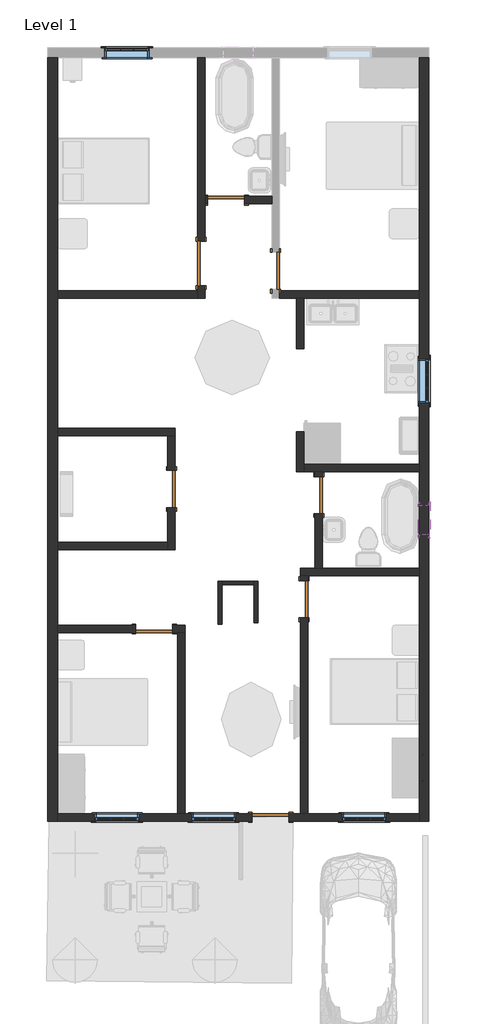
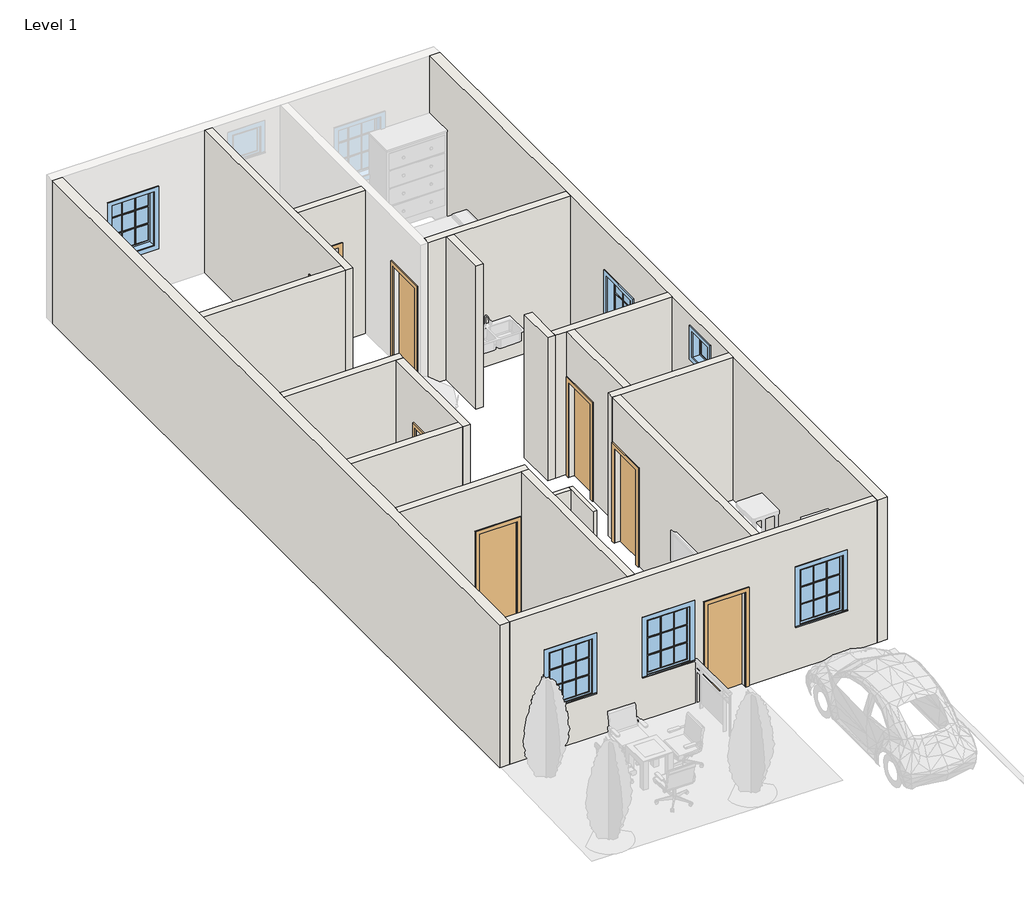
# One storey, part 1 of 2: 21 walls, 8 doors, 6 windows.
"""IFC4 building model written with IfcOpenShell, lengths in millimetres."""

from ifc_helpers import new_model, si_unit, frame, origin, origin_with_axes, place, context, project, spatial, polyline, outline, extrude, faceted_brep, transform, mapped, element, save
from components import door_255cab33, door_059fdd7e, door_686f89d2, window_29c06734, window_5c190c7e, window_e41d21a6

model = new_model("IFC4")

# Units and contexts
model_context = context("Model", 3, world=origin())
ifc_project = project(units=[si_unit("LENGTHUNIT", "METRE", prefix="MILLI")], contexts=[model_context])

# Site, building, storey
site = spatial("IfcSite", under=ifc_project)
building = spatial("IfcBuilding", under=site)
storey = spatial("IfcBuildingStorey", under=building, Name="Level 1", Elevation=0.0)

# Doors
placement = place(None, origin())
door_shape = door_255cab33(model_context)
element("IfcDoor", 1, ObjectType="Single-Flush : 30\" x 80\"", at=placement, inside=storey, context=model_context, shape_type="MappedRepresentation", body=[
    mapped(door_shape, transform((-12610.4905738, 8071.5768478, 0.0), x_axis=(-1.0, 0.0, 0.0), y_axis=(0.0, -1.0, 0.0), z_axis=(0.0, 0.0, 1.0))),
])
element("IfcDoor", 2, ObjectType="Single-Flush : 30\" x 80\"", at=placement, inside=storey, context=model_context, shape_type="MappedRepresentation", body=[
    mapped(door_shape, transform((-13728.0905738, 2153.3768478, 0.0), x_axis=(0.0, 1.0, 0.0), y_axis=(-1.0, 0.0, 0.0), z_axis=(0.0, 0.0, 1.0))),
])
element("IfcDoor", 3, ObjectType="Single-Flush : 30\" x 80\"", at=placement, inside=storey, context=model_context, shape_type="MappedRepresentation", body=[
    mapped(door_shape, transform((-10705.4905738, 2026.3768478, 0.0), x_axis=(0.0, 1.0, 0.0), y_axis=(-1.0, 0.0, 0.0), z_axis=(0.0, 0.0, 1.0))),
])
element("IfcDoor", 4, ObjectType="Single-Flush : 30\" x 80\"", at=placement, inside=storey, context=model_context, shape_type="MappedRepresentation", body=[
    mapped(door_shape, transform((-11010.2905738, -107.2231522, 0.0), x_axis=(0.0, 1.0, 0.0), y_axis=(-1.0, 0.0, 0.0), z_axis=(0.0, 0.0, 1.0))),
])
element("IfcDoor", 5, ObjectType="Single-Flush : 30\" x 80\"", at=placement, inside=storey, context=model_context, shape_type="MappedRepresentation", body=[
    mapped(door_shape, transform((-14083.6905738, -716.8231522, 0.0), x_axis=(1.0, 0.0, 0.0), y_axis=(0.0, 1.0, 0.0), z_axis=(0.0, 0.0, 1.0))),
])
door_2_shape = door_059fdd7e(model_context)
element("IfcDoor", 6, ObjectType="Single-Flush : 30\" x 80\"", at=placement, inside=storey, context=model_context, shape_type="MappedRepresentation", body=[
    mapped(door_2_shape, transform((-11594.4905738, 6623.7768478, 0.0), x_axis=(0.0, -1.0, 0.0), y_axis=(1.0, 0.0, 0.0), z_axis=(0.0, 0.0, 1.0))),
])
element("IfcDoor", 7, ObjectType="Single-Flush : 30\" x 80\"", at=placement, inside=storey, context=model_context, shape_type="MappedRepresentation", body=[
    mapped(door_2_shape, transform((-11696.0905738, -4577.6231522, 0.0), x_axis=(1.0, 0.0, 0.0), y_axis=(0.0, 1.0, 0.0), z_axis=(0.0, 0.0, 1.0))),
])
door_3_shape = door_686f89d2(model_context)
element("IfcDoor", 8, ObjectType="Single-Flush : 36\" x 84\"", at=placement, inside=storey, context=model_context, shape_type="MappedRepresentation", body=[
    mapped(door_3_shape, transform((-13118.4905738, 6776.1768478, 0.0), x_axis=(0.0, -1.0, 0.0), y_axis=(1.0, 0.0, 0.0), z_axis=(0.0, 0.0, 1.0))),
])

# Walls
element("IfcWall", 9, ObjectType="Generic - 8\"", at=placement, inside=storey, context=model_context, shape_type="Brep", body=[
    faceted_brep([(-8648.0905738, 10992.5768478, 0.0), (-8648.0905738, 6217.3768478, 0.0), (-8648.0905738, 6064.9768478, 0.0), (-8648.0905738, 2661.3768478, 0.0), (-8648.0905738, 2508.9768478, 0.0), (-8648.0905738, 527.7768478, 0.0), (-8648.0905738, 375.3768478, 0.0), (-8648.0905738, -4501.4231522, 0.0), (-8648.0905738, -4653.8231522, 0.0), (-8648.0905738, -4653.8231522, 3048.0), (-8648.0905738, -4501.4231522, 3048.0), (-8648.0905738, 375.3768478, 3048.0), (-8648.0905738, 527.7768478, 3048.0), (-8648.0905738, 2508.9768478, 3048.0), (-8648.0905738, 2661.3768478, 3048.0), (-8648.0905738, 6064.9768478, 3048.0), (-8648.0905738, 6217.3768478, 3048.0), (-8648.0905738, 10992.5768478, 3048.0), (-8648.0905738, 3905.9768478, 2133.6), (-8648.0905738, 3905.9768478, 914.4), (-8648.0905738, 4820.3768478, 914.4), (-8648.0905738, 4820.3768478, 2133.6), (-8648.0905738, 1213.5768478, 2768.6), (-8648.0905738, 1213.5768478, 2159.0), (-8648.0905738, 1823.1768478, 2159.0), (-8648.0905738, 1823.1768478, 2768.6), (-8444.8905738, 10992.5768478, 0.0), (-8444.8905738, 10992.5768478, 3048.0), (-8444.8905738, -4653.8231522, 3048.0), (-8444.8905738, -4653.8231522, 0.0), (-8444.8905738, 3905.9768478, 2133.6), (-8444.8905738, 4820.3768478, 2133.6), (-8444.8905738, 4820.3768478, 914.4), (-8444.8905738, 3905.9768478, 914.4), (-8444.8905738, 1213.5768478, 2768.6), (-8444.8905738, 1823.1768478, 2768.6), (-8444.8905738, 1823.1768478, 2159.0), (-8444.8905738, 1213.5768478, 2159.0)], [[[0, 1, 2, 3, 4, 5, 6, 7, 8, 9, 10, 11, 12, 13, 14, 15, 16, 17], [18, 19, 20, 21], [22, 23, 24, 25]], [[26, 27, 28, 29], [30, 31, 32, 33], [34, 35, 36, 37]], [[8, 7, 6, 5, 4, 3, 2, 1, 0, 26, 29]], [[0, 17, 27, 26]], [[9, 8, 29, 28]], [[19, 18, 30, 33]], [[20, 19, 33, 32]], [[21, 20, 32, 31]], [[18, 21, 31, 30]], [[23, 22, 34, 37]], [[24, 23, 37, 36]], [[25, 24, 36, 35]], [[22, 25, 35, 34]], [[17, 16, 15, 14, 13, 12, 11, 10, 9, 28, 27]]]),
])
element("IfcWall", 10, ObjectType="Generic - 8\"", at=placement, inside=storey, context=model_context, shape_type="Brep", body=[
    faceted_brep([(-16064.8905738, -4653.8231522, 0.0), (-16064.8905738, -4501.4231522, 0.0), (-16064.8905738, -793.0231522, 0.0), (-16064.8905738, -640.6231522, 0.0), (-16064.8905738, 908.7768478, 0.0), (-16064.8905738, 1061.1768478, 0.0), (-16064.8905738, 3245.5768478, 0.0), (-16064.8905738, 3397.9768478, 0.0), (-16064.8905738, 6064.9768478, 0.0), (-16064.8905738, 6217.3768478, 0.0), (-16064.8905738, 10992.5768478, 0.0), (-16064.8905738, 10992.5768478, 3048.0), (-16064.8905738, 6217.3768478, 3048.0), (-16064.8905738, 6064.9768478, 3048.0), (-16064.8905738, 3397.9768478, 3048.0), (-16064.8905738, 3245.5768478, 3048.0), (-16064.8905738, 1061.1768478, 3048.0), (-16064.8905738, 908.7768478, 3048.0), (-16064.8905738, -640.6231522, 3048.0), (-16064.8905738, -793.0231522, 3048.0), (-16064.8905738, -4501.4231522, 3048.0), (-16064.8905738, -4653.8231522, 3048.0), (-16268.0905738, -4653.8231522, 0.0), (-16268.0905738, -4653.8231522, 3048.0), (-16268.0905738, 10992.5768478, 3048.0), (-16268.0905738, 10992.5768478, 0.0)], [[[0, 1, 2, 3, 4, 5, 6, 7, 8, 9, 10, 11, 12, 13, 14, 15, 16, 17, 18, 19, 20, 21]], [[22, 23, 24, 25]], [[10, 9, 8, 7, 6, 5, 4, 3, 2, 1, 0, 22, 25]], [[11, 10, 25, 24]], [[0, 21, 23, 22]], [[21, 20, 19, 18, 17, 16, 15, 14, 13, 12, 11, 24, 23]]]),
])
element("IfcWall", 11, ObjectType="inner 3\"", at=placement, inside=storey, context=model_context, shape_type="Brep", body=[
    faceted_brep([(-12033.9549283, 261.0768478, 0.0), (-12033.9549283, 184.8768478, 0.0), (-12033.9549283, -589.8231522, 0.0), (-12033.9549283, -589.8231522, 1524.0), (-12033.9549283, 184.8768478, 1524.0), (-12033.9549283, 261.0768478, 1524.0), (-11957.7549283, 261.0768478, 0.0), (-11957.7549283, 261.0768478, 1524.0), (-11957.7549283, -589.8231522, 1524.0), (-11957.7549283, -589.8231522, 0.0)], [[[0, 1, 2, 3, 4, 5]], [[6, 7, 8, 9]], [[2, 1, 0, 6, 9]], [[3, 2, 9, 8]], [[5, 4, 3, 8, 7]], [[0, 5, 7, 6]]]),
])
element("IfcWall", 12, ObjectType="inner 3\"", at=placement, inside=storey, context=model_context, shape_type="Brep", body=[
    faceted_brep([(-12694.3549283, -615.2231522, 0.0), (-12694.3549283, 184.8768478, 0.0), (-12694.3549283, 261.0768478, 0.0), (-12694.3549283, 261.0768478, 1524.0), (-12694.3549283, 184.8768478, 1524.0), (-12694.3549283, -615.2231522, 1524.0), (-12770.5549283, -615.2231522, 0.0), (-12770.5549283, -615.2231522, 1524.0), (-12770.5549283, 261.0768478, 1524.0), (-12770.5549283, 261.0768478, 0.0)], [[[0, 1, 2, 3, 4, 5]], [[6, 7, 8, 9]], [[2, 1, 0, 6, 9]], [[5, 4, 3, 8, 7]], [[0, 5, 7, 6]], [[3, 2, 9, 8]]]),
])
element("IfcWall", 13, ObjectType="inner 3\"", at=placement, inside=storey, context=model_context, shape_type="SweptSolid", body=[
    extrude(outline(polyline([(-12033.9549283, 184.8768478), (-12694.3549283, 184.8768478), (-12694.3549283, 261.0768478), (-12033.9549283, 261.0768478), (-12033.9549283, 184.8768478)])), origin_with_axes(), (0.0, 0.0, 1.0), 1524.0),
])
element("IfcWall", 14, ObjectType="inner wall", at=placement, inside=storey, context=model_context, shape_type="Brep", body=[
    faceted_brep([(-13194.6905738, 6318.9768478, 2133.6), (-13194.6905738, 6318.9768478, 0.0), (-13194.6905738, 6217.3768478, 0.0), (-13194.6905738, 6064.9768478, 0.0), (-13194.6905738, 6064.9768478, 3048.0), (-13194.6905738, 6217.3768478, 3048.0), (-13194.6905738, 10992.5768478, 3048.0), (-13194.6905738, 10992.5768478, 0.0), (-13194.6905738, 7233.3768478, 0.0), (-13194.6905738, 7233.3768478, 2133.6), (-13042.2905738, 6064.9768478, 0.0), (-13042.2905738, 6318.9768478, 0.0), (-13042.2905738, 6318.9768478, 2133.6), (-13042.2905738, 7233.3768478, 2133.6), (-13042.2905738, 7233.3768478, 0.0), (-13042.2905738, 7995.3768478, 0.0), (-13042.2905738, 8147.7768478, 0.0), (-13042.2905738, 10992.5768478, 0.0), (-13042.2905738, 10992.5768478, 3048.0), (-13042.2905738, 8147.7768478, 3048.0), (-13042.2905738, 7995.3768478, 3048.0), (-13042.2905738, 6064.9768478, 3048.0)], [[[0, 1, 2, 3, 4, 5, 6, 7, 8, 9]], [[10, 11, 12, 13, 14, 15, 16, 17, 18, 19, 20, 21]], [[8, 7, 17, 16, 15, 14]], [[3, 2, 1, 11, 10]], [[7, 6, 18, 17]], [[4, 3, 10, 21]], [[12, 11, 1, 0]], [[13, 12, 0, 9]], [[14, 13, 9, 8]], [[6, 5, 4, 21, 20, 19, 18]]]),
])
element("IfcWall", 15, ObjectType="inner wall", at=placement, inside=storey, context=model_context, shape_type="SweptSolid", body=[
    extrude(outline(polyline([(-16064.8905738, 6217.3768478), (-13194.6905738, 6217.3768478), (-13194.6905738, 6064.9768478), (-16064.8905738, 6064.9768478), (-16064.8905738, 6217.3768478)])), origin_with_axes(), (0.0, 0.0, 1.0), 3048.0),
])
element("IfcWall", 16, ObjectType="inner wall", at=placement, inside=storey, context=model_context, shape_type="Brep", body=[
    faceted_brep([(-11518.2905738, 6064.9768478, 0.0), (-11162.6905738, 6064.9768478, 0.0), (-11010.2905738, 6064.9768478, 0.0), (-8648.0905738, 6064.9768478, 0.0), (-8648.0905738, 6064.9768478, 3048.0), (-11010.2905738, 6064.9768478, 3048.0), (-11162.6905738, 6064.9768478, 3048.0), (-11518.2905738, 6064.9768478, 3048.0), (-11518.2905738, 6217.3768478, 0.0), (-11518.2905738, 6217.3768478, 3048.0), (-8648.0905738, 6217.3768478, 3048.0), (-8648.0905738, 6217.3768478, 0.0)], [[[0, 1, 2, 3, 4, 5, 6, 7]], [[8, 9, 10, 11]], [[3, 2, 1, 0, 8, 11]], [[0, 7, 9, 8]], [[4, 3, 11, 10]], [[7, 6, 5, 4, 10, 9]]]),
])
element("IfcWall", 17, ObjectType="inner wall", at=placement, inside=storey, context=model_context, shape_type="SweptSolid", body=[
    extrude(outline(polyline([(0.0, -13042.2905738), (0.0, -12991.4905738), (2032.0, -12991.4905738), (2032.0, -12229.4905738), (0.0, -12229.4905738), (0.0, -11670.6905738), (3048.0, -11670.6905738), (3048.0, -13042.2905738), (0.0, -13042.2905738)])), frame((0.0, 7995.3768478, 0.0), z_axis=(0.0, 1.0, 0.0), x_axis=(0.0, 0.0, 1.0)), (0.0, 0.0, 1.0), 152.4),
])
element("IfcWall", 18, ObjectType="inner wall", at=placement, inside=storey, context=model_context, shape_type="Brep", body=[
    faceted_brep([(-16064.8905738, 3245.5768478, 0.0), (-13804.2905738, 3245.5768478, 0.0), (-13651.8905738, 3245.5768478, 0.0), (-13651.8905738, 3245.5768478, 3048.0), (-13804.2905738, 3245.5768478, 3048.0), (-16064.8905738, 3245.5768478, 3048.0), (-16064.8905738, 3397.9768478, 0.0), (-16064.8905738, 3397.9768478, 3048.0), (-13651.8905738, 3397.9768478, 3048.0), (-13651.8905738, 3397.9768478, 0.0)], [[[0, 1, 2, 3, 4, 5]], [[6, 7, 8, 9]], [[2, 1, 0, 6, 9]], [[0, 5, 7, 6]], [[3, 2, 9, 8]], [[5, 4, 3, 8, 7]]]),
])
element("IfcWall", 19, ObjectType="inner wall", at=placement, inside=storey, context=model_context, shape_type="Brep", body=[
    faceted_brep([(-13804.2905738, 3245.5768478, 0.0), (-13804.2905738, 2534.3768478, 0.0), (-13804.2905738, 2534.3768478, 2032.0), (-13804.2905738, 1772.3768478, 2032.0), (-13804.2905738, 1772.3768478, 0.0), (-13804.2905738, 1061.1768478, 0.0), (-13804.2905738, 908.7768478, 0.0), (-13804.2905738, 908.7768478, 3048.0), (-13804.2905738, 1061.1768478, 3048.0), (-13804.2905738, 3245.5768478, 3048.0), (-13651.8905738, 2534.3768478, 2032.0), (-13651.8905738, 2534.3768478, 0.0), (-13651.8905738, 3245.5768478, 0.0), (-13651.8905738, 3245.5768478, 3048.0), (-13651.8905738, 908.7768478, 3048.0), (-13651.8905738, 908.7768478, 0.0), (-13651.8905738, 1772.3768478, 0.0), (-13651.8905738, 1772.3768478, 2032.0)], [[[0, 1, 2, 3, 4, 5, 6, 7, 8, 9]], [[10, 11, 12, 13, 14, 15, 16, 17]], [[16, 15, 6, 5, 4]], [[12, 11, 1, 0]], [[0, 9, 13, 12]], [[7, 6, 15, 14]], [[2, 1, 11, 10]], [[3, 2, 10, 17]], [[4, 3, 17, 16]], [[9, 8, 7, 14, 13]]]),
])
element("IfcWall", 20, ObjectType="inner wall", at=placement, inside=storey, context=model_context, shape_type="SweptSolid", body=[
    extrude(outline(polyline([(-16064.8905738, 1061.1768478), (-13804.2905738, 1061.1768478), (-13804.2905738, 908.7768478), (-16064.8905738, 908.7768478), (-16064.8905738, 1061.1768478)])), origin_with_axes(), (0.0, 0.0, 1.0), 3048.0),
])
element("IfcWall", 21, ObjectType="inner wall", at=placement, inside=storey, context=model_context, shape_type="Brep", body=[
    faceted_brep([(-13702.6905738, -793.0231522, 2032.0), (-13702.6905738, -793.0231522, 0.0), (-13601.0905738, -793.0231522, 0.0), (-13448.6905738, -793.0231522, 0.0), (-13448.6905738, -793.0231522, 3048.0), (-13601.0905738, -793.0231522, 3048.0), (-16064.8905738, -793.0231522, 3048.0), (-16064.8905738, -793.0231522, 0.0), (-14464.6905738, -793.0231522, 0.0), (-14464.6905738, -793.0231522, 2032.0), (-13448.6905738, -640.6231522, 0.0), (-13702.6905738, -640.6231522, 0.0), (-13702.6905738, -640.6231522, 2032.0), (-14464.6905738, -640.6231522, 2032.0), (-14464.6905738, -640.6231522, 0.0), (-16064.8905738, -640.6231522, 0.0), (-16064.8905738, -640.6231522, 3048.0), (-13448.6905738, -640.6231522, 3048.0)], [[[0, 1, 2, 3, 4, 5, 6, 7, 8, 9]], [[10, 11, 12, 13, 14, 15, 16, 17]], [[8, 7, 15, 14]], [[3, 2, 1, 11, 10]], [[7, 6, 16, 15]], [[4, 3, 10, 17]], [[12, 11, 1, 0]], [[13, 12, 0, 9]], [[14, 13, 9, 8]], [[6, 5, 4, 17, 16]]]),
])
element("IfcWall", 22, ObjectType="inner wall", at=placement, inside=storey, context=model_context, shape_type="SweptSolid", body=[
    extrude(outline(polyline([(-13601.0905738, -4501.4231522), (-13601.0905738, -793.0231522), (-13448.6905738, -793.0231522), (-13448.6905738, -4501.4231522), (-13601.0905738, -4501.4231522)])), origin_with_axes(), (0.0, 0.0, 1.0), 3048.0),
])
element("IfcWall", 23, ObjectType="inner wall", at=placement, inside=storey, context=model_context, shape_type="Brep", body=[
    faceted_brep([(-8648.0905738, -4501.4231522, 0.0), (-10934.0905738, -4501.4231522, 0.0), (-11086.4905738, -4501.4231522, 0.0), (-11315.0905738, -4501.4231522, 0.0), (-11315.0905738, -4501.4231522, 2032.0), (-12077.0905738, -4501.4231522, 2032.0), (-12077.0905738, -4501.4231522, 0.0), (-13448.6905738, -4501.4231522, 0.0), (-13601.0905738, -4501.4231522, 0.0), (-16064.8905738, -4501.4231522, 0.0), (-16064.8905738, -4501.4231522, 3048.0), (-13601.0905738, -4501.4231522, 3048.0), (-13448.6905738, -4501.4231522, 3048.0), (-11086.4905738, -4501.4231522, 3048.0), (-10934.0905738, -4501.4231522, 3048.0), (-8648.0905738, -4501.4231522, 3048.0), (-10235.5905738, -4501.4231522, 2133.6), (-10235.5905738, -4501.4231522, 914.4), (-9321.1905738, -4501.4231522, 914.4), (-9321.1905738, -4501.4231522, 2133.6), (-13321.6905738, -4501.4231522, 2133.6), (-13321.6905738, -4501.4231522, 914.4), (-12407.2905738, -4501.4231522, 914.4), (-12407.2905738, -4501.4231522, 2133.6), (-15302.8905738, -4501.4231522, 2133.6), (-15302.8905738, -4501.4231522, 914.4), (-14388.4905738, -4501.4231522, 914.4), (-14388.4905738, -4501.4231522, 2133.6), (-11315.0905738, -4653.8231522, 2032.0), (-11315.0905738, -4653.8231522, 0.0), (-8648.0905738, -4653.8231522, 0.0), (-8648.0905738, -4653.8231522, 3048.0), (-16064.8905738, -4653.8231522, 3048.0), (-16064.8905738, -4653.8231522, 0.0), (-12077.0905738, -4653.8231522, 0.0), (-12077.0905738, -4653.8231522, 2032.0), (-10235.5905738, -4653.8231522, 2133.6), (-9321.1905738, -4653.8231522, 2133.6), (-9321.1905738, -4653.8231522, 914.4), (-10235.5905738, -4653.8231522, 914.4), (-13321.6905738, -4653.8231522, 2133.6), (-12407.2905738, -4653.8231522, 2133.6), (-12407.2905738, -4653.8231522, 914.4), (-13321.6905738, -4653.8231522, 914.4), (-15302.8905738, -4653.8231522, 2133.6), (-14388.4905738, -4653.8231522, 2133.6), (-14388.4905738, -4653.8231522, 914.4), (-15302.8905738, -4653.8231522, 914.4)], [[[0, 1, 2, 3, 4, 5, 6, 7, 8, 9, 10, 11, 12, 13, 14, 15], [16, 17, 18, 19], [20, 21, 22, 23], [24, 25, 26, 27]], [[28, 29, 30, 31, 32, 33, 34, 35], [36, 37, 38, 39], [40, 41, 42, 43], [44, 45, 46, 47]], [[34, 33, 9, 8, 7, 6]], [[30, 29, 3, 2, 1, 0]], [[4, 3, 29, 28]], [[5, 4, 28, 35]], [[6, 5, 35, 34]], [[0, 15, 31, 30]], [[17, 16, 36, 39]], [[18, 17, 39, 38]], [[19, 18, 38, 37]], [[16, 19, 37, 36]], [[21, 20, 40, 43]], [[22, 21, 43, 42]], [[23, 22, 42, 41]], [[20, 23, 41, 40]], [[25, 24, 44, 47]], [[26, 25, 47, 46]], [[27, 26, 46, 45]], [[24, 27, 45, 44]], [[10, 9, 33, 32]], [[15, 14, 13, 12, 11, 10, 32, 31]]]),
])
element("IfcWall", 24, ObjectType="inner wall", at=placement, inside=storey, context=model_context, shape_type="SweptSolid", body=[
    extrude(outline(polyline([(-11162.6905738, 5023.5768478), (-11162.6905738, 6064.9768478), (-11010.2905738, 6064.9768478), (-11010.2905738, 5023.5768478), (-11162.6905738, 5023.5768478)])), origin_with_axes(), (0.0, 0.0, 1.0), 3048.0),
])
element("IfcWall", 25, ObjectType="inner wall", at=placement, inside=storey, context=model_context, shape_type="Brep", body=[
    faceted_brep([(-11010.2905738, 2508.9768478, 0.0), (-10781.6905738, 2508.9768478, 0.0), (-10629.2905738, 2508.9768478, 0.0), (-8648.0905738, 2508.9768478, 0.0), (-8648.0905738, 2508.9768478, 3048.0), (-10629.2905738, 2508.9768478, 3048.0), (-10781.6905738, 2508.9768478, 3048.0), (-11010.2905738, 2508.9768478, 3048.0), (-11010.2905738, 2661.3768478, 0.0), (-11010.2905738, 2661.3768478, 3048.0), (-8648.0905738, 2661.3768478, 3048.0), (-8648.0905738, 2661.3768478, 0.0)], [[[0, 1, 2, 3, 4, 5, 6, 7]], [[8, 9, 10, 11]], [[3, 2, 1, 0, 8, 11]], [[0, 7, 9, 8]], [[4, 3, 11, 10]], [[7, 6, 5, 4, 10, 9]]]),
])
element("IfcWall", 26, ObjectType="inner wall", at=placement, inside=storey, context=model_context, shape_type="SweptSolid", body=[
    extrude(outline(polyline([(2508.9768478, 0.0), (2407.3768478, 0.0), (2407.3768478, 2032.0), (1645.3768478, 2032.0), (1645.3768478, 0.0), (527.7768478, 0.0), (527.7768478, 3048.0), (2508.9768478, 3048.0), (2508.9768478, 0.0)])), frame((-10781.6905738, 0.0, 0.0), z_axis=(1.0, 0.0, 0.0), x_axis=(0.0, 1.0, 0.0)), (0.0, 0.0, 1.0), 152.4),
])
element("IfcWall", 27, ObjectType="inner wall", at=placement, inside=storey, context=model_context, shape_type="Brep", body=[
    faceted_brep([(-11086.4905738, 375.3768478, 0.0), (-10934.0905738, 375.3768478, 0.0), (-8648.0905738, 375.3768478, 0.0), (-8648.0905738, 375.3768478, 3048.0), (-10934.0905738, 375.3768478, 3048.0), (-11086.4905738, 375.3768478, 3048.0), (-11086.4905738, 527.7768478, 0.0), (-11086.4905738, 527.7768478, 3048.0), (-10781.6905738, 527.7768478, 3048.0), (-10629.2905738, 527.7768478, 3048.0), (-8648.0905738, 527.7768478, 3048.0), (-8648.0905738, 527.7768478, 0.0), (-10629.2905738, 527.7768478, 0.0), (-10781.6905738, 527.7768478, 0.0)], [[[0, 1, 2, 3, 4, 5]], [[6, 7, 8, 9, 10, 11, 12, 13]], [[2, 1, 0, 6, 13, 12, 11]], [[3, 2, 11, 10]], [[0, 5, 7, 6]], [[5, 4, 3, 10, 9, 8, 7]]]),
])
element("IfcWall", 28, ObjectType="inner wall", at=placement, inside=storey, context=model_context, shape_type="SweptSolid", body=[
    extrude(outline(polyline([(375.3768478, 0.0), (273.7768478, 0.0), (273.7768478, 2032.0), (-488.2231522, 2032.0), (-488.2231522, 0.0), (-4501.4231522, 0.0), (-4501.4231522, 3048.0), (375.3768478, 3048.0), (375.3768478, 0.0)])), frame((-11086.4905738, 0.0, 0.0), z_axis=(1.0, 0.0, 0.0), x_axis=(0.0, 1.0, 0.0)), (0.0, 0.0, 1.0), 152.4),
])
element("IfcWall", 29, ObjectType="inner wall", at=placement, inside=storey, context=model_context, shape_type="Brep", body=[
    faceted_brep([(-11162.6905738, 3321.7768478, 0.0), (-11162.6905738, 2508.9768478, 0.0), (-11162.6905738, 2508.9768478, 3048.0), (-11162.6905738, 3321.7768478, 3048.0), (-11010.2905738, 3321.7768478, 0.0), (-11010.2905738, 3321.7768478, 3048.0), (-11010.2905738, 2661.3768478, 3048.0), (-11010.2905738, 2508.9768478, 3048.0), (-11010.2905738, 2508.9768478, 0.0), (-11010.2905738, 2661.3768478, 0.0)], [[[0, 1, 2, 3]], [[4, 5, 6, 7, 8, 9]], [[1, 0, 4, 9, 8]], [[0, 3, 5, 4]], [[2, 1, 8, 7]], [[3, 2, 7, 6, 5]]]),
])

# Windows
window_shape = window_29c06734(model_context)
element("IfcWindow", 30, ObjectType="Casement 3x3 with Trim : 36\" x 48\"", at=placement, inside=storey, context=model_context, shape_type="MappedRepresentation", body=[
    mapped(window_shape, transform((-14642.4905738, 11094.1768478, 0.0), x_axis=(1.0, 0.0, 0.0), y_axis=(0.0, 1.0, 0.0), z_axis=(0.0, 0.0, 1.0))),
])
element("IfcWindow", 31, ObjectType="Casement 3x3 with Trim : 36\" x 48\"", at=placement, inside=storey, context=model_context, shape_type="MappedRepresentation", body=[
    mapped(window_shape, transform((-8546.4905738, 4363.1768478, 0.0), x_axis=(0.0, -1.0, 0.0), y_axis=(1.0, 0.0, 0.0), z_axis=(0.0, 0.0, 1.0))),
])
window_2_shape = window_5c190c7e(model_context)
element("IfcWindow", 32, ObjectType="Casement 3x3 with Trim : 36\" x 48\"", at=placement, inside=storey, context=model_context, shape_type="MappedRepresentation", body=[
    mapped(window_2_shape, transform((-9778.3905738, -4577.6231522, 0.0), x_axis=(-1.0, 0.0, 0.0), y_axis=(0.0, -1.0, 0.0), z_axis=(0.0, 0.0, 1.0))),
])
element("IfcWindow", 33, ObjectType="Casement 3x3 with Trim : 36\" x 48\"", at=placement, inside=storey, context=model_context, shape_type="MappedRepresentation", body=[
    mapped(window_2_shape, transform((-12864.4905738, -4577.6231522, 0.0), x_axis=(-1.0, 0.0, 0.0), y_axis=(0.0, -1.0, 0.0), z_axis=(0.0, 0.0, 1.0))),
])
element("IfcWindow", 34, ObjectType="Casement 3x3 with Trim : 36\" x 48\"", at=placement, inside=storey, context=model_context, shape_type="MappedRepresentation", body=[
    mapped(window_2_shape, transform((-14845.6905738, -4577.6231522, 0.0), x_axis=(-1.0, 0.0, 0.0), y_axis=(0.0, -1.0, 0.0), z_axis=(0.0, 0.0, 1.0))),
])
window_3_shape = window_e41d21a6(model_context)
element("IfcWindow", 35, ObjectType="Transom with Trim : 24\" x 24\"", at=placement, inside=storey, context=model_context, shape_type="MappedRepresentation", body=[
    mapped(window_3_shape, transform((-8546.4905738, 1480.2768478, 0.0), x_axis=(0.0, -1.0, 0.0), y_axis=(1.0, 0.0, 0.0), z_axis=(0.0, 0.0, 1.0))),
])

save(model, "model.ifc")

# Revit data of these elements
# Type "Single-Flush : 30\" x 80\""
#   Type Mark = "5"
#   Construction Type Id = "MDOOR"
#   Assembly Code = "C1020"
#   Analytic Construction = "Metal"
#   Thickness = 0' - 2"
#   Heat Transfer Coefficient (U) = 0.651978 BTU/(h·ft²·°F)
#   Height = 6' - 8"
#   Trim Projection Ext = 0' - 1"
#   Trim Projection Int = 0' - 1"
#   Trim Width = 0' - 3"
#   Width = 2' - 6"
#   Define Thermal Properties by = 1
#   Door Material = Door - Panel
#   Frame Material = Door - Frame
#   Visual Light Transmittance = 0
#   Solar Heat Gain Coefficient = 0
#   Function = (empty or 0)
#   Wall Closure = (empty or 0)
# Type "Single-Flush : 36\" x 84\""
#   Type Mark = "1"
#   Construction Type Id = "MDOOR"
#   Assembly Code = "C1020"
#   Analytic Construction = "Metal"
#   Thickness = 0' - 2"
#   Heat Transfer Coefficient (U) = 0.651978 BTU/(h·ft²·°F)
#   Height = 7' - 0"
#   Trim Projection Ext = 0' - 1"
#   Trim Projection Int = 0' - 1"
#   Trim Width = 0' - 3"
#   Width = 3' - 0"
#   Define Thermal Properties by = 1
#   Door Material = Door - Panel
#   Frame Material = Door - Frame
#   Visual Light Transmittance = 0
#   Solar Heat Gain Coefficient = 0
#   Function = (empty or 0)
#   Wall Closure = (empty or 0)
# Type "Generic - 8\""
#   Assembly Code = "B2010"
#   Layers, outside or top first: 0' - 8" "Brick, Common" (function 1)
# Type "inner 3\""
#   Assembly Code = "B2010"
#   Layers, outside or top first: 0' - 3" "Brick, Common" (function 1)
# Type "inner wall"
#   Assembly Code = "B2010"
#   Layers, outside or top first: 0' - 6" "Brick, Common" (function 1)
# Type "Casement 3x3 with Trim : 36\" x 48\""
#   Type Mark = "10"
#   Construction Type Id = "GSP4R"
#   Assembly Code = "B2020100"
#   Analytic Construction = "1/8 in Pilkington single glazing"
#   Visual Light Transmittance = 0.9
#   Solar Heat Gain Coefficient = 0.78
#   Heat Transfer Coefficient (U) = 0.6496 BTU/(h·ft²·°F)
#   Height = 4' - 0"
#   Default Sill Height = 3' - 0"
#   Trim Projection - Ext. = 0' - 0 1/2"
#   Trim Projection - Int. = 0' - 0 3/4"
#   Trim Width - Exterior = 0' - 3 1/2"
#   Trim Width - Interior = 0' - 3 1/2"
#   Width = 3' - 0"
#   Window Inset = 0' - 0 3/4"
#   Define Thermal Properties by = 1
#   Glass Pane Material = Glass
#   Sash Material = Sash
#   Trim Exterior Material = Trim
#   Trim Interior Material = Trim
#   Wall Closure = (empty or 0)
# Type "Transom with Trim : 24\" x 24\""
#   Type Mark = "13"
#   Construction Type Id = "GSP4R"
#   Assembly Code = "B2020100"
#   Analytic Construction = "1/8 in Pilkington single glazing"
#   Visual Light Transmittance = 0.9
#   Solar Heat Gain Coefficient = 0.78
#   Heat Transfer Coefficient (U) = 0.6496 BTU/(h·ft²·°F)
#   Height = 2' - 0"
#   Default Sill Height = 7' - 1"
#   Trim Projection - Ext. = 0' - 0 1/2"
#   Trim Projection - Int. = 0' - 0 3/4"
#   Trim Width - Exterior = 0' - 3 1/2"
#   Trim Width - Interior = 0' - 3 1/2"
#   Width = 2' - 0"
#   Window Inset = 0' - 0 3/4"
#   Define Thermal Properties by = 1
#   Glass Pane Material = Glass
#   Sash Material = Sash
#   Trim Exterior Material = Trim
#   Trim Interior Material = Trim
#   Wall Closure = (empty or 0)
# Elements 1, 2, 3, 4, 5, 6, 7 (IfcDoor, "Single-Flush : 30\" x 80\"")
#   Phase Created = New Construction
#   Materials on its faces: "Door - Frame", "Door - Panel"
# Element 8 (IfcDoor, "Single-Flush : 36\" x 84\"")
#   Phase Created = New Construction
#   Materials on its faces: "Door - Frame", "Door - Panel"
# Elements 9, 10 (IfcWall, "Generic - 8\"")
#   Top Offset = 0' - 0"
#   Base Offset = 0' - 0"
#   Unconnected Height = 10' - 0"
#   wall height = 10' - 0"
#   Phase Created = New Construction
#   Base Constraint = Level 1
#   Materials on its faces: "Brick, Common"
# Elements 11, 12, 13 (IfcWall, "inner 3\"")
#   Top Offset = 0' - 0"
#   Base Offset = 0' - 0"
#   Unconnected Height = 5' - 0"
#   wall height = 5' - 0"
#   Phase Created = New Construction
#   Base Constraint = Level 1
#   Materials on its faces: "Brick, Common"
# Elements 14, 15, 16, 17, 18, 19, 20, 21, 22, 23, 24, 25, 26, 27, 28, 29 (IfcWall, "inner wall")
#   Top Offset = 0' - 0"
#   Base Offset = 0' - 0"
#   Unconnected Height = 10' - 0"
#   wall height = 10' - 0"
#   Phase Created = New Construction
#   Base Constraint = Level 1
#   Materials on its faces: "Brick, Common"
# Element 30 (IfcWindow, "Casement 3x3 with Trim : 36\" x 48\"")
#   Mark = "1"
#   Phase Created = New Construction
#   Materials on its faces: "Sash", "Glass", "Trim"
# Element 31 (IfcWindow, "Casement 3x3 with Trim : 36\" x 48\"")
#   Mark = "3"
#   Phase Created = New Construction
#   Materials on its faces: "Sash", "Glass", "Trim"
# Element 32 (IfcWindow, "Casement 3x3 with Trim : 36\" x 48\"")
#   Mark = "4"
#   Phase Created = New Construction
#   Materials on its faces: "Sash", "Glass", "Trim"
# Element 33 (IfcWindow, "Casement 3x3 with Trim : 36\" x 48\"")
#   Mark = "5"
#   Phase Created = New Construction
#   Materials on its faces: "Sash", "Glass", "Trim"
# Element 34 (IfcWindow, "Casement 3x3 with Trim : 36\" x 48\"")
#   Mark = "6"
#   Phase Created = New Construction
#   Materials on its faces: "Sash", "Glass", "Trim"
# Element 35 (IfcWindow, "Transom with Trim : 24\" x 24\"")
#   Mark = "7"
#   Phase Created = New Construction
#   Materials on its faces: "Sash", "Trim", "Glass"
# Materials
#   "Door - Panel": class "Wood", colour RGB 210 159 95, transparency 0
#   "Door - Frame": colour RGB 118 70 51, transparency 0
#   "Brick, Common": class "Masonry", colour RGB 170 98 104, transparency 0, Description = "Common brick", Cost = 0
#   "Glass": class "Glass", colour RGB 0 128 192, transparency 0.75, Description = "Soda Lime Glass", Cost = 0
#   "Sash": class "Wood", colour RGB 224 178 126, transparency 0
#   "Trim": class "Wood", colour RGB 224 178 126, transparency 0
# Room at (-14600.339, 9093.075) mm, phase "New Construction", upper level "Level 1", upper offset 10' - 0", lower offset 0' - 0"
#   Number = "1"
#   Name = "BEDROOM"
# Room at (-12307.869, 9792.882) mm, phase "New Construction", upper level "Level 1", upper offset 10' - 0", lower offset 0' - 0"
#   Number = "2"
#   Name = "TOILET"
# Room at (-9991.269, -6905.947) mm, phase "New Construction", upper level "Level 1", upper offset 10' - 0", lower offset 0' - 0"
#   Number = "12"
#   Name = "PARKING"
# Room at (-9991.269, 8530.726) mm, phase "New Construction", upper level "Level 1", upper offset 10' - 0", lower offset 0' - 0"
#   Number = "3"
#   Name = "BEDROOM"
# Room at (-12307.869, 3977.249) mm, phase "New Construction", upper level "Level 1", upper offset 10' - 0", lower offset 0' - 0"
#   Number = "4"
#   Name = "DINING"
# Room at (-14914.045, 2022.617) mm, phase "New Construction", upper level "Level 1", upper offset 10' - 0", lower offset 0' - 0"
#   Number = "5"
#   Name = "STORE"
# Room at (-9991.269, 4677.056) mm, phase "New Construction", upper level "Level 1", upper offset 10' - 0", lower offset 0' - 0"
#   Number = "6"
#   Name = "KITCHEN"
# Room at (-9460.381, 1491.73) mm, phase "New Construction", upper level "Level 1", upper offset 10' - 0", lower offset 0' - 0"
#   Number = "7"
#   Name = "TOILET"
# Room at (-14914.045, -2827.765) mm, phase "New Construction", upper level "Level 1", upper offset 10' - 0", lower offset 0' - 0"
#   Number = "8"
#   Name = "BEDROOM"
# Room at (-12307.869, -2321.009) mm, phase "New Construction", upper level "Level 1", upper offset 10' - 0", lower offset 0' - 0"
#   Number = "9"
#   Name = "LIVING"
# Room at (-9991.269, -1934.909) mm, phase "New Construction", upper level "Level 1", upper offset 10' - 0", lower offset 0' - 0"
#   Number = "10"
#   Name = "BEDROOM"
# Room at (-14136.669, -6375.06) mm, phase "New Construction", upper level "Level 1", upper offset 10' - 0", lower offset 0' - 0"
#   Number = "11"
#   Name = "VERANDAH"
# Room at (-12307.869, -389.396) mm, phase "New Construction", upper level "Level 1", upper offset 10' - 0", lower offset 0' - 0"
#   Number = "13"
